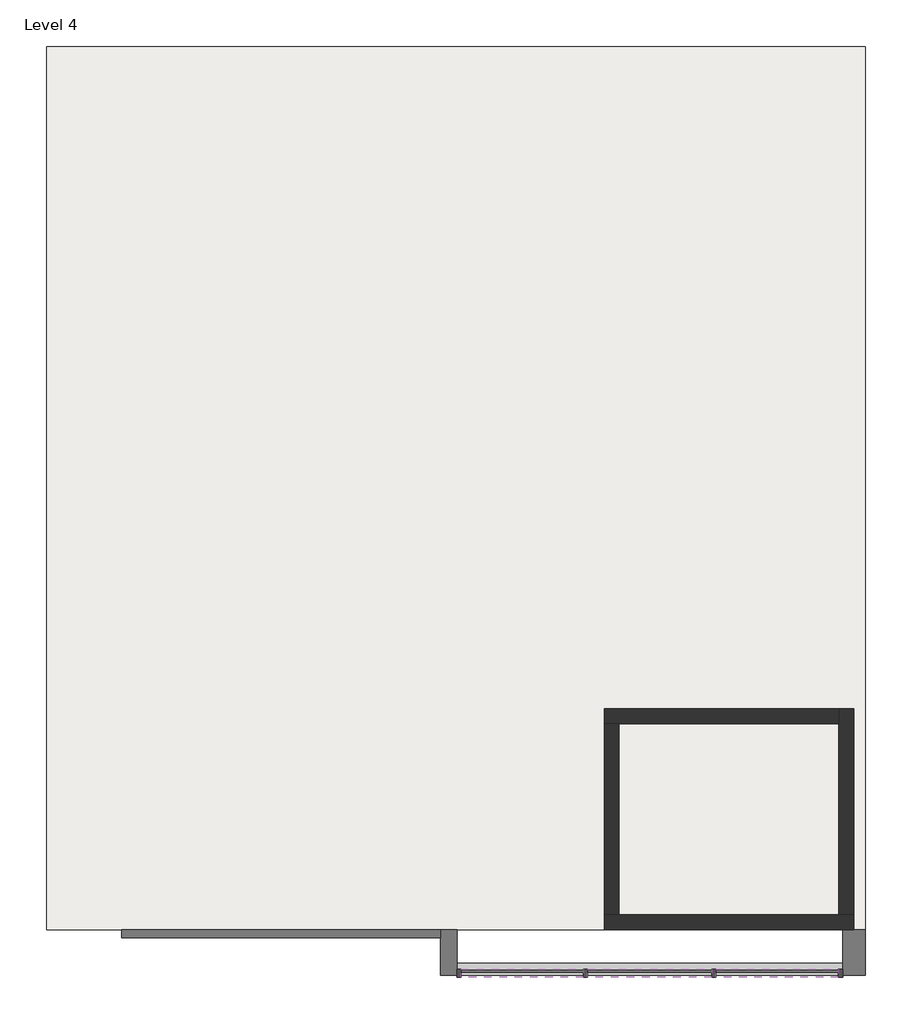
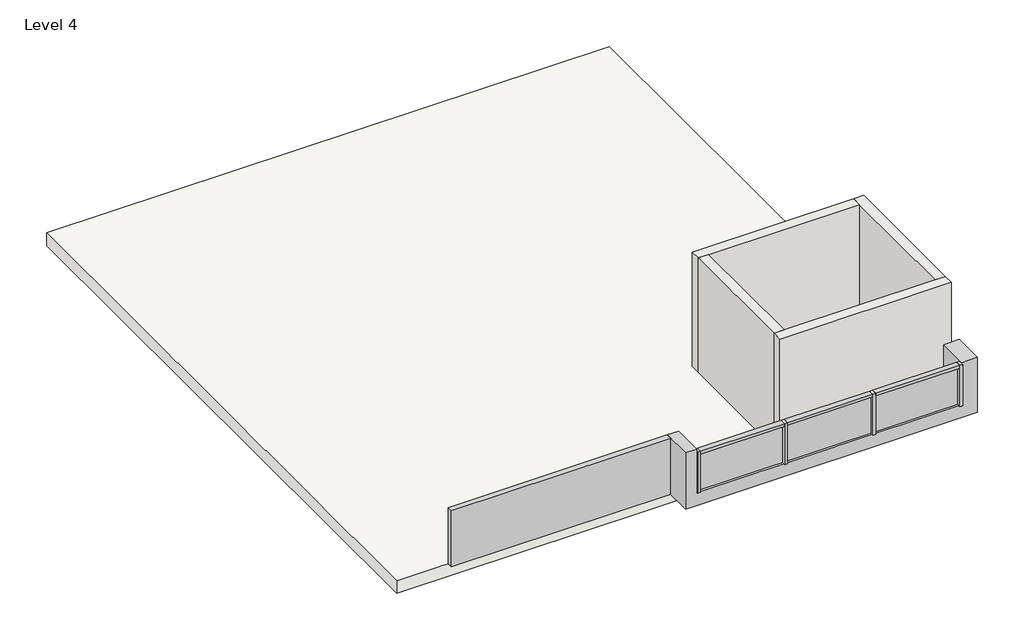
# One storey: 7 members, 4 walls, 3 plates, 2 proxies, 1 roof.
"""IFC4 building model written with IfcOpenShell, lengths in millimetres."""

from ifc_helpers import new_model, si_unit, frame, origin, place, context, project, spatial, polyline, outline, extrude, faceted_brep, transform, mapped, element, save
from components import generic_models_6_generic_models_6_46bcb04b, generic_models_7_generic_models_7_06ca3c93, member_9fb0cd34, member_e7372dc0, member_11fc1043, member_7f5bebbe, system_panel_glazed_090522f0, system_panel_glazed_6e11b836

model = new_model("IFC4")

# Units and contexts
model_context = context("Model", 3, world=origin())
ifc_project = project(units=[si_unit("LENGTHUNIT", "METRE", prefix="MILLI")], contexts=[model_context])

# Site, building, storey
site = spatial("IfcSite", under=ifc_project)
building = spatial("IfcBuilding", under=site)
storey = spatial("IfcBuildingStorey", under=building, Name="Level 4", Elevation=9144.0)

# Proxies
placement = place(None, origin())
generic_models_6_generic_models_6_shape = generic_models_6_generic_models_6_46bcb04b(model_context)
element("IfcBuildingElementProxy", 1, Name="Generic Models 6 : Generic Models 6", ObjectType="Generic Models 6 : Generic Models 6", at=placement, inside=storey, context=model_context, shape_type="MappedRepresentation", body=[
    mapped(generic_models_6_generic_models_6_shape, transform((0.0, 0.0, 0.0), x_axis=(1.0, 0.0, 0.0), y_axis=(0.0, 1.0, 0.0), z_axis=(0.0, 0.0, 1.0))),
])
generic_models_7_generic_models_7_shape = generic_models_7_generic_models_7_06ca3c93(model_context)
element("IfcBuildingElementProxy", 2, Name="Generic Models 7 : Generic Models 7", ObjectType="Generic Models 7 : Generic Models 7", at=placement, inside=storey, context=model_context, shape_type="MappedRepresentation", body=[
    mapped(generic_models_7_generic_models_7_shape, transform((0.0, 0.0, 0.0), x_axis=(1.0, 0.0, 0.0), y_axis=(0.0, 1.0, 0.0), z_axis=(0.0, 0.0, 1.0))),
])

# Members
member_shape = member_9fb0cd34(model_context)
element("IfcMember", 3, ObjectType="Rectangular Mullion : 2.5\" x 5\" rectangular", at=placement, inside=storey, context=model_context, shape_type="MappedRepresentation", body=[
    mapped(member_shape, transform((-10622.3081241, -14813.9130528, 9753.6), x_axis=(1.0, 0.0, 0.0), y_axis=(0.0, -1.0, 0.0), z_axis=(0.0, 0.0, -1.0))),
])
element("IfcMember", 4, ObjectType="Rectangular Mullion : 2.5\" x 5\" rectangular", at=placement, inside=storey, context=model_context, shape_type="MappedRepresentation", body=[
    mapped(member_shape, transform((-8624.1747908, -14813.9130528, 9753.6), x_axis=(1.0, 0.0, 0.0), y_axis=(0.0, -1.0, 0.0), z_axis=(0.0, 0.0, -1.0))),
])
member_2_shape = member_e7372dc0(model_context)
element("IfcMember", 5, ObjectType="Rectangular Mullion : 2.5\" x 5\" rectangular", at=placement, inside=storey, context=model_context, shape_type="MappedRepresentation", body=[
    mapped(member_2_shape, transform((-8655.9247908, -14813.9130528, 10736.6943516), x_axis=(0.0, 0.0, 1.0), y_axis=(0.0, -1.0, 0.0), z_axis=(1.0, 0.0, 0.0))),
])
member_3_shape = member_11fc1043(model_context)
element("IfcMember", 6, ObjectType="Rectangular Mullion : 2.5\" x 5\" rectangular", at=placement, inside=storey, context=model_context, shape_type="MappedRepresentation", body=[
    mapped(member_3_shape, transform((-10654.0581241, -14813.9130528, 10736.6943516), x_axis=(0.0, 0.0, 1.0), y_axis=(0.0, -1.0, 0.0), z_axis=(1.0, 0.0, 0.0))),
])
element("IfcMember", 7, ObjectType="Rectangular Mullion : 2.5\" x 5\" rectangular", at=placement, inside=storey, context=model_context, shape_type="MappedRepresentation", body=[
    mapped(member_3_shape, transform((-6689.5414575, -14813.9130528, 10736.6943516), x_axis=(0.0, 0.0, 1.0), y_axis=(0.0, -1.0, 0.0), z_axis=(1.0, 0.0, 0.0))),
])
member_4_shape = member_7f5bebbe(model_context)
element("IfcMember", 8, ObjectType="Rectangular Mullion : 2.5\" x 5\" rectangular", at=placement, inside=storey, context=model_context, shape_type="MappedRepresentation", body=[
    mapped(member_4_shape, transform((-6626.0414575, -14813.9130528, 9753.6), x_axis=(1.0, 0.0, 0.0), y_axis=(0.0, -1.0, 0.0), z_axis=(0.0, 0.0, -1.0))),
])
element("IfcMember", 9, ObjectType="Rectangular Mullion : 2.5\" x 5\" rectangular", at=placement, inside=storey, context=model_context, shape_type="MappedRepresentation", body=[
    mapped(member_4_shape, transform((-12620.4414575, -14813.9130528, 10736.6943516), x_axis=(-1.0, 0.0, 0.0), y_axis=(0.0, -1.0, 0.0), z_axis=(0.0, 0.0, 1.0))),
])

# Plates
system_panel_glazed_shape = system_panel_glazed_090522f0(model_context)
element("IfcPlate", 10, ObjectType="System Panel : Glazed", at=placement, inside=storey, context=model_context, shape_type="MappedRepresentation", body=[
    mapped(system_panel_glazed_shape, transform((-9623.2414575, -14813.9130528, 9753.6), x_axis=(1.0, 0.0, 0.0), y_axis=(0.0, 1.0, 0.0), z_axis=(0.0, 0.0, 1.0))),
])
system_panel_glazed_2_shape = system_panel_glazed_6e11b836(model_context)
element("IfcPlate", 11, ObjectType="System Panel : Glazed", at=placement, inside=storey, context=model_context, shape_type="MappedRepresentation", body=[
    mapped(system_panel_glazed_2_shape, transform((-11605.4997908, -14813.9130528, 9753.6), x_axis=(1.0, 0.0, 0.0), y_axis=(0.0, 1.0, 0.0), z_axis=(0.0, 0.0, 1.0))),
])
element("IfcPlate", 12, ObjectType="System Panel : Glazed", at=placement, inside=storey, context=model_context, shape_type="MappedRepresentation", body=[
    mapped(system_panel_glazed_2_shape, transform((-7640.9831241, -14813.9130528, 9753.6), x_axis=(1.0, 0.0, 0.0), y_axis=(0.0, 1.0, 0.0), z_axis=(0.0, 0.0, 1.0))),
])

# Roof
element("IfcRoof", 13, ObjectType="Generic - 12\"", at=placement, inside=storey, context=model_context, shape_type="SweptSolid", body=[
    extrude(outline(polyline([(-18997.6195233, -418.7752569), (-6272.2195233, -418.7752569), (-6272.2195233, -14134.7752569), (-18997.6195233, -14134.7752569), (-18997.6195233, -418.7752569)])), frame((0.0, 0.0, 9144.0), z_axis=(0.0, 0.0, 1.0), x_axis=(1.0, 0.0, 0.0)), (0.0, 0.0, 1.0), 304.8),
])

# Walls
element("IfcWall", 14, ObjectType="9\"", at=placement, inside=storey, context=model_context, shape_type="Brep", body=[
    faceted_brep([(-10329.8695233, -14134.7752569, 9144.0), (-6454.240816, -14134.7752569, 9144.0), (-6454.240816, -14134.7752569, 12192.0), (-10329.8695233, -14134.7752569, 12192.0), (-10329.8695233, -13906.1752569, 9144.0), (-10329.8695233, -13906.1752569, 12192.0), (-10101.2695233, -13906.1752569, 12192.0), (-6682.840816, -13906.1752569, 12192.0), (-6454.240816, -13906.1752569, 12192.0), (-6454.240816, -13906.1752569, 9144.0), (-6682.840816, -13906.1752569, 9144.0), (-10101.2695233, -13906.1752569, 9144.0)], [[[0, 1, 2, 3]], [[4, 5, 6, 7, 8, 9, 10, 11]], [[1, 0, 4, 11, 10, 9]], [[3, 2, 8, 7, 6, 5]], [[2, 1, 9, 8]], [[0, 3, 5, 4]]]),
])
element("IfcWall", 15, ObjectType="9\"", at=placement, inside=storey, context=model_context, shape_type="Brep", body=[
    faceted_brep([(-6454.240816, -13906.1752569, 9144.0), (-6454.240816, -10705.7752569, 9144.0), (-6454.240816, -10705.7752569, 12192.0), (-6454.240816, -13906.1752569, 12192.0), (-6682.840816, -13906.1752569, 9144.0), (-6682.840816, -13906.1752569, 12192.0), (-6682.840816, -10934.3752569, 12192.0), (-6682.840816, -10705.7752569, 12192.0), (-6682.840816, -10705.7752569, 9144.0), (-6682.840816, -10934.3752569, 9144.0)], [[[0, 1, 2, 3]], [[4, 5, 6, 7, 8, 9]], [[1, 0, 4, 9, 8]], [[3, 2, 7, 6, 5]], [[0, 3, 5, 4]], [[2, 1, 8, 7]]]),
])
element("IfcWall", 16, ObjectType="9\"", at=placement, inside=storey, context=model_context, shape_type="Brep", body=[
    faceted_brep([(-6682.840816, -10705.7752569, 9144.0), (-10329.8695233, -10705.7752569, 9144.0), (-10329.8695233, -10705.7752569, 12192.0), (-6682.840816, -10705.7752569, 12192.0), (-6682.840816, -10934.3752569, 9144.0), (-6682.840816, -10934.3752569, 12192.0), (-10101.2695233, -10934.3752569, 12192.0), (-10329.8695233, -10934.3752569, 12192.0), (-10329.8695233, -10934.3752569, 9144.0), (-10101.2695233, -10934.3752569, 9144.0)], [[[0, 1, 2, 3]], [[4, 5, 6, 7, 8, 9]], [[1, 0, 4, 9, 8]], [[3, 2, 7, 6, 5]], [[0, 3, 5, 4]], [[2, 1, 8, 7]]]),
])
element("IfcWall", 17, ObjectType="9\"", at=placement, inside=storey, context=model_context, shape_type="SweptSolid", body=[
    extrude(outline(polyline([(-10329.8695233, -13906.1752569), (-10329.8695233, -10934.3752569), (-10101.2695233, -10934.3752569), (-10101.2695233, -13906.1752569), (-10329.8695233, -13906.1752569)])), frame((0.0, 0.0, 9144.0), z_axis=(0.0, 0.0, 1.0), x_axis=(1.0, 0.0, 0.0)), (0.0, 0.0, 1.0), 3048.0),
])

save(model, "model.ifc")

# Revit data of these elements
# Type "Rectangular Mullion : 2.5\" x 5\" rectangular"
#   built-in parameter 1007304 = 0.416667 (stored number, unit not read)
#   built-in parameter 1007301 = 0.104167 (stored number, unit not read)
#   built-in parameter 1007300 = 0.104167 (stored number, unit not read)
# Type "System Panel : Glazed"
#   Construction Type Id = "GSP4R"
#   Analytic Construction = "1/8 in Pilkington single glazing"
#   Visual Light Transmittance = 0.9
#   Solar Heat Gain Coefficient = 0.86
#   Heat Transfer Coefficient (U) = 1.18115 BTU/(h·ft²·°F)
#   Define Thermal Properties by = 1
# Type "Generic - 12\""
#   Assembly Code = "B1020"
#   Layers, outside or top first: 1' - 0" no material (function 1)
# Type "9\""
#   Assembly Code = "B2010"
#   Layers, outside or top first: 0' - 9" no material (function 1)
# Element 1 (IfcBuildingElementProxy, "Generic Models 6 : Generic Models 6")
#   Phase Created = New Construction
# Element 2 (IfcBuildingElementProxy, "Generic Models 7 : Generic Models 7")
#   Phase Created = New Construction
# Elements 3, 4, 5, 6, 7, 8, 9 (IfcMember, "Rectangular Mullion : 2.5\" x 5\" rectangular")
#   Phase Created = New Construction
#   Materials on its faces: "Aluminum"
# Elements 10, 11, 12 (IfcPlate, "System Panel : Glazed")
#   Phase Created = New Construction
#   Materials on its faces: "Glass"
# Element 13 (IfcRoof, "Generic - 12\"")
#   built-in parameter 1001705 = 31 (stored number, unit not read)
#   built-in parameter 1001710 = 33615
#   Phase Created = New Construction
#   Materials on its faces: "Default Roof"
# Elements 14, 15, 16, 17 (IfcWall, "9\"")
#   Top Offset = 0' - 0"
#   Base Offset = 0' - 0"
#   Unconnected Height = 10' - 0"
#   wall height = 10' - 0"
#   Phase Created = New Construction
#   Base Constraint = Level 4
#   Materials on its faces: "Default Wall"
# Materials
#   "Aluminum": class "Metal", colour RGB 247 247 247, transparency 0, Description = "Aluminum 6061", Cost = 0
#   "Glass": class "Glass", colour RGB 0 128 192, transparency 0.75, Description = "Soda Lime Glass", Cost = 0
#   "Default Roof": colour RGB 88 101 114, transparency 0, Cost = 0
#   "Default Wall": colour RGB 128 128 128, transparency 0, Cost = 0
